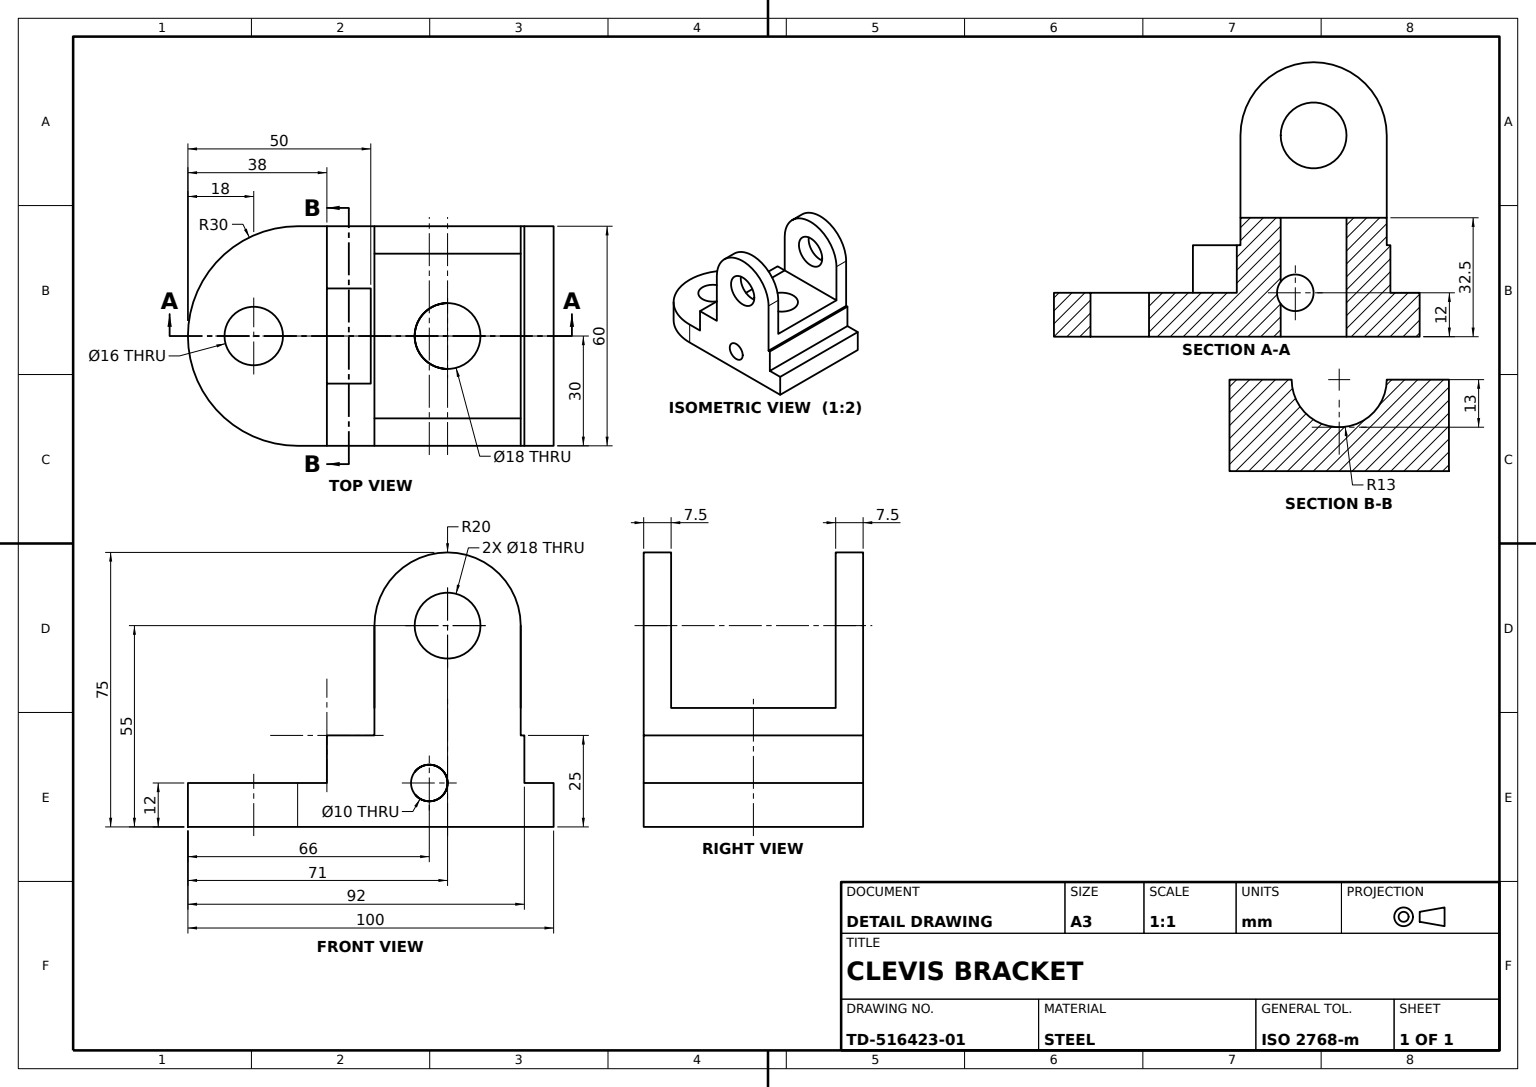
from build123d import *

# Parameters (mm, degrees)
BASE_PLATE_DEPTH              = 12
BASE_HOLE_DEPTH               = 12
UPRIGHT_BLOCK_SKETCH_W        = 42
UPRIGHT_BLOCK_SKETCH_H        = 12
UPRIGHT_BLOCK_DEPTH           = 60
CLEVIS_EAR_DEPTH              = 7.5
CLEVIS_EAR_EXTENSION_SKETCH_W = 45
CLEVIS_EAR_EXTENSION_SKETCH_H = 40
CLEVIS_EAR_EXTENSION_DEPTH    = 7.5
CLEVIS_PIN_BORE_SKETCH_R      = 9
CLEVIS_PIN_BORE_DEPTH         = 90.5
SADDLE_BLOCK_SKETCH_W         = 12
SADDLE_BLOCK_SKETCH_H         = 13
SADDLE_BLOCK_DEPTH            = 60
SADDLE_CUT_SKETCH_R           = 13
SADDLE_CUT_DEPTH              = 12
THROUGH_HOLE_A_SKETCH_R       = 9
THROUGH_HOLE_A_DEPTH          = 139
THROUGH_HOLE_B_SKETCH_R       = 5
THROUGH_HOLE_B_DEPTH          = 139
THROUGH_HOLE_C_SKETCH_R       = 8
THROUGH_HOLE_C_DEPTH          = 139


with BuildPart() as part:
    # Base Plate Sketch → Base Plate (new body)
    with BuildSketch(Plane(origin=(0, 0, 0), x_dir=(1, 0, 0), z_dir=(0, 1, 0))):
        Polygon((0, 0), (30, 0), (30, 100), (-30, 100), (-30, 0), align=None)
    extrude(amount=BASE_PLATE_DEPTH)

    # Base Hole Sketch → Base Hole (cut)
    with BuildSketch(Plane(origin=(0, 12, 0), x_dir=(1, 0, 0), z_dir=(0, 1, 0))):
        with BuildLine():
            ThreePointArc((1.57e-07, 0), (-21.21320338, 8.786796509), (-30, 30))
            Line((-30, 30), (-30, 0))
            Line((-30, 0), (1.57e-07, 0))
        make_face()
        with BuildLine():
            Line((30, 0), (30, 30))
            ThreePointArc((30, 30), (21.213203491, 8.78679662), (1.57e-07, 0))
            Line((1.57e-07, 0), (30, 0))
        make_face()
    extrude(amount=-BASE_HOLE_DEPTH, mode=Mode.SUBTRACT)

    # Upright Block Sketch → Upright Block (add)
    with BuildSketch(Plane(origin=(30, 0, 0), x_dir=(0, 0, -1), z_dir=(1, 0, 0))):
        Polygon((50, 12), (92, 12), (92, 25), (62, 25), (50, 25), align=None)
        with Locations((71, 6)):
            Rectangle(UPRIGHT_BLOCK_SKETCH_W, UPRIGHT_BLOCK_SKETCH_H)
    extrude(amount=-UPRIGHT_BLOCK_DEPTH)

    # Clevis Ear Sketch → Clevis Ear (add)
    with BuildSketch(Plane.ZY.offset(30)):
        with BuildLine():
            Line((-51, 55), (-51, 25))
            Line((-51, 25), (-91, 25))
            Line((-91, 25), (-91, 55))
            ThreePointArc((-91, 55), (-71, 75), (-51, 55))
        make_face()
    clevis_ear = extrude(amount=-CLEVIS_EAR_DEPTH)

    # Clevis Ear Mirror: Clevis Ear across plane
    add(clevis_ear.mirror(Plane(origin=(0, 0, 0), x_dir=(0, 0, 1), z_dir=(1, 0, 0))))

    # Clevis Ear Extension Sketch → Clevis Ear Extension (add)
    with BuildSketch(Plane(origin=(0, 25, 0), x_dir=(1, 0, 0), z_dir=(0, 1, 0))):
        with Locations((0, 71)):
            Rectangle(CLEVIS_EAR_EXTENSION_SKETCH_W, CLEVIS_EAR_EXTENSION_SKETCH_H)
    extrude(amount=CLEVIS_EAR_EXTENSION_DEPTH)

    # Clevis Pin Bore Sketch → Clevis Pin Bore (cut)
    with BuildSketch(Plane(origin=(0, 32.5, 0), x_dir=(1, 0, 0), z_dir=(0, 1, 0))):
        with Locations(Location((0, 71, 0), (0, 0, 270))):
            Circle(CLEVIS_PIN_BORE_SKETCH_R)
    extrude(amount=-CLEVIS_PIN_BORE_DEPTH, mode=Mode.SUBTRACT)

    # Saddle Block Sketch → Saddle Block (add)
    with BuildSketch(Plane(origin=(30, 0, 0), x_dir=(0, 0, -1), z_dir=(1, 0, 0))):
        with Locations((44, 18.5)):
            Rectangle(SADDLE_BLOCK_SKETCH_W, SADDLE_BLOCK_SKETCH_H)
    extrude(amount=-SADDLE_BLOCK_DEPTH)

    # Saddle Cut Sketch → Saddle Cut (cut)
    with BuildSketch(Plane.XY.offset(-38)):
        with Locations((0, 25)):
            Circle(SADDLE_CUT_SKETCH_R)
    extrude(amount=-SADDLE_CUT_DEPTH, mode=Mode.SUBTRACT)

    # Through Hole A Sketch → Through Hole A (cut)
    with BuildSketch(Plane.ZY.offset(30)):
        with Locations((-71, 55)):
            Circle(THROUGH_HOLE_A_SKETCH_R)
    extrude(amount=-THROUGH_HOLE_A_DEPTH, mode=Mode.SUBTRACT)

    # Through Hole B Sketch → Through Hole B (cut)
    with BuildSketch(Plane.ZY.offset(30)):
        with Locations((-66, 12)):
            Circle(THROUGH_HOLE_B_SKETCH_R)
    extrude(amount=-THROUGH_HOLE_B_DEPTH, mode=Mode.SUBTRACT)

    # Through Hole C Sketch → Through Hole C (cut)
    with BuildSketch(Plane(origin=(0, 12, 0), x_dir=(1, 0, 0), z_dir=(0, 1, 0))):
        with Locations(Location((0, 18, 0), (0, 0, 270))):
            Circle(THROUGH_HOLE_C_SKETCH_R)
    extrude(amount=-THROUGH_HOLE_C_DEPTH, mode=Mode.SUBTRACT)


solid = part.part
